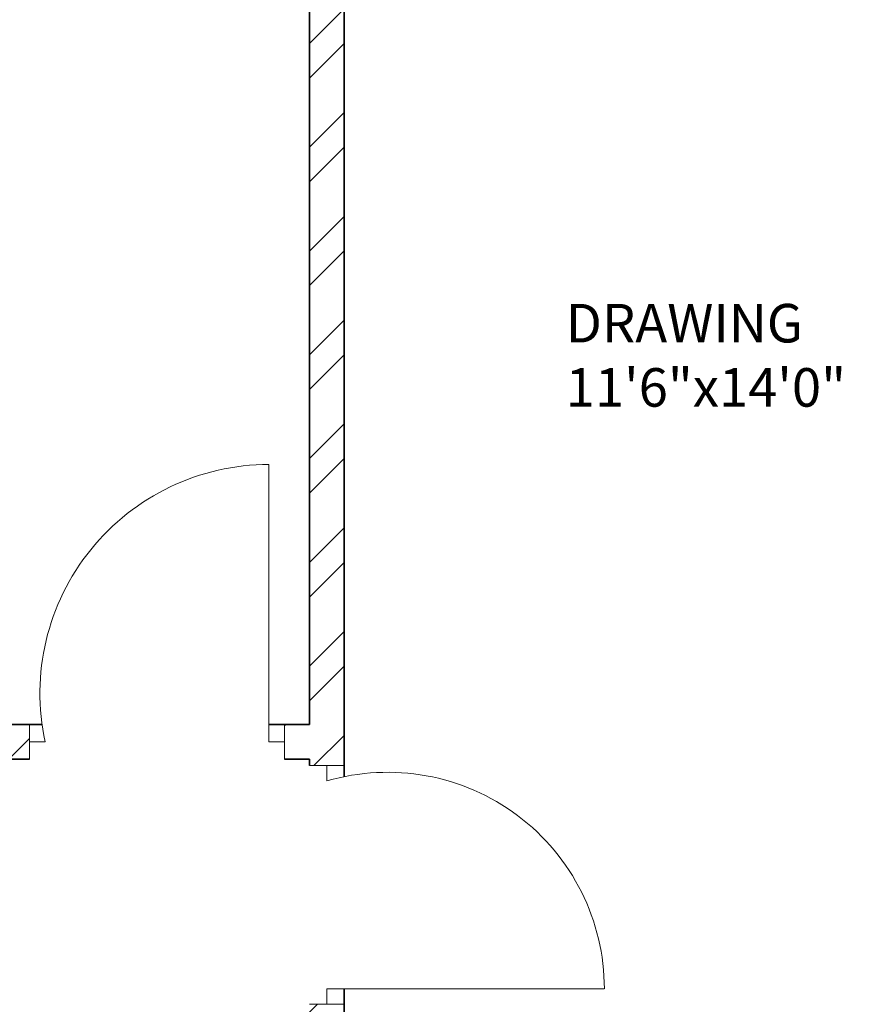
# Model space of a CAD drawing. Units: inches. Extents: x 1885 to 2748, y 783 to 2421.
# Tile 101 of 117: x 2449 to 2557, y 1850 to 1977. Entities that reach past the tile are written whole.
import ezdxf

# ---------------------------------------------------------------- set-up
doc = ezdxf.new("R2010")
doc.units = ezdxf.units.IN
for name, color, linetype, lineweight in [('A-AREA-IDEN', 7, 'Continuous', 18), ('A-DOOR', 31, 'Continuous', 18), ('A-WALL', 7, 'Continuous', 35)]:
    doc.layers.add(name, color=color, linetype=linetype, lineweight=lineweight)
doc.layers.add('A-WALL-PATT', color=85, linetype='Continuous', lineweight=13, true_color=0x58ba48)
doc.styles.get("Standard").update_dxf_attribs({"font": 'arial.ttf'})

msp = doc.modelspace()

# ---------------------------------------------------------------- hatches: boundary and pattern name
at = {"layer": 'A-WALL-PATT'}
h = msp.add_hatch(dxfattribs=at)
h.set_pattern_fill('ANSI32', color=256)
h.paths.add_polyline_path([(2007.77, 2318.01), (1980.77, 2318.01), (1980.77, 2281.22), (1985.27, 2281.22), (1985.27, 2313.51), (2007.77, 2313.51), (2007.77, 2315.76)])
h.paths.add_polyline_path([(2094.32, 2318.01), (2067.77, 2318.01), (2067.77, 2313.51), (2094.32, 2313.51), (2094.32, 2315.76)])
h.paths.add_polyline_path([(2131.37, 2315.76), (2131.37, 2318.01), (2131.19, 2318.01), (2112.61, 2318.01), (2112.61, 2313.51), (2117.27, 2313.51), (2117.27, 2255.2), (2121.77, 2255.2), (2121.77, 2313.51), (2131.37, 2313.51)])
h.paths.add_polyline_path([(2190.51, 2318.01), (2155.37, 2318.01), (2155.37, 2313.51), (2169.77, 2313.51), (2169.77, 2229.51), (2121.77, 2229.51), (2121.77, 2233.45), (2119.52, 2233.45), (2117.27, 2233.45), (2117.27, 2201.1), (2121.77, 2201.1), (2121.77, 2225.01), (2169.77, 2225.01), (2169.77, 2165.01), (2306.27, 2165.01), (2306.27, 2066.01), (2310.77, 2066.01), (2344.27, 2066.01), (2486.27, 2066.01), (2486.27, 1886.01), (2483.02, 1886.01), (2483.02, 1881.51), (2486.27, 1881.51), (2486.27, 1880.68), (2490.77, 1880.68), (2490.77, 2070.51), (2344.27, 2070.51), (2310.77, 2070.51), (2310.77, 2165.01), (2310.77, 2173.64), (2308.52, 2173.64), (2306.27, 2173.64), (2306.27, 2169.51), (2174.27, 2169.51), (2174.27, 2313.51), (2190.51, 2313.51), (2190.51, 2315.76)])
h.paths.add_polyline_path([(1985.27, 2221.22), (1980.77, 2221.22), (1980.77, 2165.01), (1992.77, 2165.01), (1992.77, 2141.93), (1997.27, 2141.93), (1997.27, 2165.01), (2117.27, 2165.01), (2117.27, 2163.13), (2121.77, 2163.13), (2121.77, 2172.73), (2119.52, 2172.73), (2117.27, 2172.73), (2117.27, 2169.51), (1985.27, 2169.51)])
h.paths.add_polyline_path([(1997.27, 2105.93), (1992.77, 2105.93), (1992.77, 2070.51), (2016.77, 2070.51), (2016.77, 2059.12), (2019.02, 2059.12), (2021.27, 2059.12), (2021.27, 2070.51), (2117.27, 2070.51), (2117.27, 2022.51), (2114.42, 2022.51), (2114.42, 2018.01), (2123.63, 2018.01), (2123.63, 2020.26), (2123.63, 2022.51), (2121.77, 2022.51), (2121.77, 2142.59), (2119.52, 2142.59), (2117.27, 2142.59), (2117.27, 2075.01), (1997.27, 2075.01)])
h.paths.add_polyline_path([(2092.03, 2020.26), (2092.03, 2022.51), (2021.27, 2022.51), (2021.27, 2035.12), (2016.77, 2035.12), (2016.77, 2018.01), (2016.77, 1978.78), (2021.27, 1978.78), (2021.27, 2018.01), (2092.03, 2018.01)])
h.paths.add_polyline_path([(2260.94, 2022.51), (2153.1, 2022.51), (2153.1, 2020.26), (2153.1, 2018.01), (2155.27, 2018.01), (2155.27, 1886.01), (2107.63, 1886.01), (2107.63, 1881.51), (2182.91, 1881.51), (2182.91, 1883.76), (2182.91, 1886.01), (2159.77, 1886.01), (2159.77, 2018.01), (2260.94, 2018.01), (2260.94, 2020.26)])
h.paths.add_polyline_path([(2047.63, 1883.76), (2047.63, 1886.01), (2021.27, 1886.01), (2021.27, 1918.78), (2019.02, 1918.78), (2016.77, 1918.78), (2016.77, 1881.51), (2047.63, 1881.51)])
h.paths.add_polyline_path([(2306.36, 1883.76), (2306.36, 1886.01), (2296.27, 1886.01), (2296.27, 1982.01), (2316.54, 1982.01), (2316.54, 1984.26), (2316.54, 1986.51), (2296.27, 1986.51), (2296.27, 2022.51), (2289.28, 2022.51), (2289.28, 2018.01), (2291.77, 2018.01), (2291.77, 1886.01), (2242.91, 1886.01), (2242.91, 1881.51), (2306.36, 1881.51)], flags=17)
h.paths.add_polyline_path([(1985.27, 1843.01), (2021.6, 1843.01), (2021.53, 1845.44), (2021.48, 1847.51), (1980.77, 1847.51), (1980.77, 1809.45), (1985.27, 1809.45)])
h.paths.add_polyline_path([(2131.48, 1845.26), (2131.48, 1847.51), (2081.53, 1847.51), (2081.53, 1843.01), (2117.27, 1843.01), (2117.27, 1784.15), (2119.52, 1784.15), (2121.77, 1784.15), (2121.77, 1843.01), (2131.48, 1843.01)])
h.paths.add_polyline_path([(2203.89, 1847.51), (2155.48, 1847.51), (2155.48, 1843.01), (2169.77, 1843.01), (2169.77, 1759.01), (2121.77, 1759.01), (2121.77, 1761.46), (2117.27, 1761.46), (2117.27, 1730.43), (2121.77, 1730.43), (2121.77, 1754.51), (2177.42, 1754.51), (2177.42, 1756.76), (2177.42, 1759.01), (2174.27, 1759.01), (2174.27, 1843.01), (2203.89, 1843.01)])
h.paths.add_polyline_path([(2335.55, 1845.26), (2335.55, 1847.51), (2239.89, 1847.51), (2239.89, 1843.01), (2306.27, 1843.01), (2306.27, 1759.01), (2199.49, 1759.01), (2199.49, 1754.51), (2310.77, 1754.51), (2310.77, 1843.01), (2335.55, 1843.01)])
h.paths.add_polyline_path([(2348.77, 2022.51), (2344.27, 2022.51), (2344.27, 1986.51), (2341.68, 1986.51), (2341.68, 1982.01), (2344.27, 1982.01), (2344.27, 1886.01), (2330.36, 1886.01), (2330.36, 1881.51), (2361.63, 1881.51), (2361.63, 1883.76), (2361.63, 1886.01), (2348.77, 1886.01)], flags=17)
h.paths.add_polyline_path([(2283.25, 2315.76), (2283.25, 2318.01), (2238.51, 2318.01), (2238.51, 2313.51), (2283.25, 2313.51)], flags=17)
h.paths.add_polyline_path([(2363.27, 2348.01), (2388.68, 2348.01), (2388.68, 2350.26), (2388.68, 2352.51), (2358.77, 2352.51), (2358.77, 2348.01), (2358.77, 2318.01), (2344.48, 2318.01), (2344.48, 2313.51), (2358.77, 2313.51), (2358.77, 2229.51), (2310.77, 2229.51), (2310.77, 2231.95), (2306.27, 2231.95), (2306.27, 2205.61), (2310.77, 2205.61), (2310.77, 2225.01), (2358.77, 2225.01), (2358.77, 2211.51), (2452.33, 2211.51), (2452.33, 2213.76), (2452.33, 2216.01), (2363.27, 2216.01), (2363.27, 2318.01)])
h.paths.add_polyline_path([(2310.77, 2313.51), (2320.48, 2313.51), (2320.48, 2315.76), (2320.48, 2318.01), (2302.73, 2318.01), (2302.73, 2313.51), (2306.27, 2313.51), (2306.27, 2251.08), (2310.77, 2251.08)], flags=17)
h.paths.add_polyline_path([(2490.77, 2352.51), (2486.27, 2352.51), (2448.68, 2352.51), (2448.68, 2348.01), (2486.27, 2348.01), (2486.27, 2318.01), (2486.27, 2216.01), (2481.78, 2216.01), (2481.78, 2211.51), (2486.27, 2211.51), (2486.27, 2165.01), (2493.29, 2165.01), (2493.29, 2167.26), (2493.29, 2169.51), (2490.77, 2169.51), (2490.77, 2313.51), (2494.43, 2313.51), (2494.43, 2318.01), (2490.77, 2318.01)])
h.paths.add_polyline_path([(2534.65, 2318.01), (2515.69, 2318.01), (2515.69, 2313.51), (2534.65, 2313.51), (2534.65, 2315.76)])
h.paths.add_polyline_path([(2618.27, 2318.01), (2594.65, 2318.01), (2594.65, 2313.51), (2613.77, 2313.51), (2613.77, 2281.71), (2618.27, 2281.71)])
h.paths.add_polyline_path([(2618.27, 2221.71), (2613.77, 2221.71), (2613.77, 2169.51), (2554.02, 2169.51), (2554.02, 2165.01), (2613.77, 2165.01), (2613.77, 2152.88), (2618.27, 2152.88)])
h.paths.add_polyline_path([(2618.27, 2128.88), (2616.02, 2128.88), (2613.77, 2128.88), (2613.77, 2117.01), (2529.77, 2117.01), (2529.77, 2165.01), (2532.85, 2165.01), (2532.85, 2169.51), (2522.87, 2169.51), (2522.87, 2165.01), (2525.27, 2165.01), (2525.27, 2117.01), (2525.27, 2112.51), (2525.27, 2108.58), (2529.77, 2108.58), (2529.77, 2112.51), (2613.77, 2112.51), (2613.77, 2080.19), (2618.27, 2080.19)])
h.paths.add_polyline_path([(2618.27, 2044.19), (2616.02, 2044.19), (2613.77, 2044.19), (2613.77, 2015.51), (2529.77, 2015.51), (2529.77, 2088.58), (2527.52, 2088.58), (2525.27, 2088.58), (2525.27, 2011.01), (2613.77, 2011.01), (2613.77, 1956.75), (2618.27, 1956.75)])
h.paths.add_polyline_path([(2618.27, 1881.51), (2618.27, 1896.75), (2613.77, 1896.75), (2613.77, 1881.51), (2613.77, 1847.51), (2592.71, 1847.51), (2592.71, 1843.01), (2613.77, 1843.01), (2613.77, 1765.01), (2613.77, 1760.51), (2609.62, 1760.51), (2609.62, 1756.01), (2613.77, 1756.01), (2613.77, 1660.01), (2608.54, 1660.01), (2608.54, 1655.51), (2613.77, 1655.51), (2613.77, 1508.16), (2618.27, 1508.16)])
h.paths.add_polyline_path([(2565.77, 1843.01), (2569, 1843.01), (2569, 1847.51), (2490.77, 1847.51), (2490.77, 1849.7), (2488.52, 1849.7), (2486.27, 1849.7), (2486.27, 1847.51), (2477.27, 1847.51), (2477.27, 1838.51), (2477.27, 1821.49), (2486.27, 1821.49), (2486.27, 1838.51), (2561.27, 1838.51), (2561.27, 1765.01), (2486.27, 1765.01), (2486.27, 1786.16), (2477.27, 1786.16), (2477.27, 1765.01), (2477.27, 1756.01), (2486.27, 1756.01), (2565.77, 1756.01), (2585.62, 1756.01), (2585.62, 1758.26), (2585.62, 1760.51), (2565.77, 1760.51), (2565.77, 1765.01)])
h.paths.add_polyline_path([(2486.27, 1651.01), (2561.27, 1651.01), (2561.27, 1567.01), (2486.27, 1567.01), (2486.27, 1591.32), (2477.27, 1591.32), (2477.27, 1567.01), (2477.27, 1558.01), (2477.27, 1555.44), (2481.77, 1555.44), (2481.77, 1558.01), (2568.65, 1558.01), (2568.65, 1560.26), (2568.65, 1562.51), (2565.77, 1562.51), (2565.77, 1655.51), (2584.54, 1655.51), (2584.54, 1657.76), (2584.54, 1660.01), (2565.77, 1660.01), (2486.27, 1660.01), (2477.27, 1660.01), (2477.27, 1651.01), (2477.27, 1632.99), (2486.27, 1632.99)])
h.paths.add_polyline_path([(2449.97, 1883.76), (2449.97, 1886.01), (2421.63, 1886.01), (2421.63, 1881.51), (2449.97, 1881.51)], flags=17)
h.paths.add_polyline_path([(2447.27, 1847.51), (2395.55, 1847.51), (2395.55, 1843.01), (2442.77, 1843.01), (2442.77, 1809.27), (2447.27, 1809.27)])
h.paths.add_polyline_path([(1985.27, 1749.45), (1980.77, 1749.45), (1980.77, 1694.5), (1985.27, 1694.5), (1985.27, 1694.51), (1986.9, 1694.51), (1986.9, 1697.78), (1986.9, 1699.01), (1985.27, 1699.01)])
h.paths.add_polyline_path([(2152.77, 1699.01), (2121.77, 1699.01), (2121.77, 1703.67), (2119.52, 1703.67), (2117.27, 1703.67), (2117.27, 1699.01), (2009.22, 1699.01), (2009.22, 1694.51), (2148.27, 1694.51), (2148.27, 1692.63), (2152.77, 1692.63)])
h.paths.add_polyline_path([(2016.27, 1694.51), (2011.77, 1694.51), (2011.77, 1558.01), (2040.81, 1558.01), (2040.81, 1560.26), (2040.81, 1562.51), (2016.27, 1562.51)])
h.paths.add_polyline_path([(2152.77, 1663.02), (2150.52, 1663.02), (2148.27, 1663.02), (2148.27, 1562.51), (2100.81, 1562.51), (2100.81, 1558.01), (2165.12, 1558.01), (2165.12, 1560.26), (2165.12, 1562.51), (2152.77, 1562.51), (2152.77, 1610.51), (2224.77, 1610.51), (2224.77, 1607.99), (2229.27, 1607.99), (2229.27, 1615.01), (2152.77, 1615.01)])
h.paths.add_polyline_path([(2238.61, 1560.26), (2238.61, 1562.51), (2229.27, 1562.51), (2229.27, 1588.76), (2227.02, 1588.76), (2224.77, 1588.77), (2224.77, 1562.51), (2189.12, 1562.51), (2189.12, 1558.01), (2238.61, 1558.01)])
h.paths.add_polyline_path([(2336.02, 1560.26), (2336.02, 1562.51), (2310.77, 1562.51), (2310.77, 1656.35), (2308.52, 1656.35), (2306.27, 1656.35), (2306.27, 1562.51), (2286.61, 1562.51), (2286.61, 1558.01), (2336.02, 1558.01)])
h.paths.add_polyline_path([(2447.27, 1690.97), (2445.02, 1690.97), (2442.77, 1690.97), (2442.77, 1687.01), (2306.27, 1687.01), (2306.27, 1680.75), (2310.77, 1680.75), (2310.77, 1682.51), (2442.77, 1682.51), (2442.77, 1562.51), (2396.02, 1562.51), (2396.02, 1558.01), (2447.27, 1558.01)])
h.paths.add_polyline_path([(2447.27, 1749.27), (2445.02, 1749.27), (2442.77, 1749.27), (2442.77, 1717.23), (2447.27, 1717.23)])
h.paths.add_polyline_path([(2044.67, 1521.76), (2044.67, 1524.01), (2007.27, 1524.01), (2007.27, 1503.49), (2009.52, 1503.49), (2011.77, 1503.49), (2011.77, 1519.51), (2044.67, 1519.51)])
h.paths.add_polyline_path([(2177.97, 1521.76), (2177.97, 1524.01), (2104.67, 1524.01), (2104.67, 1519.51), (2145.77, 1519.51), (2145.77, 1387.51), (2143.37, 1387.51), (2143.37, 1383.01), (2251.59, 1383.01), (2251.59, 1385.26), (2251.59, 1387.51), (2150.27, 1387.51), (2150.27, 1519.51), (2177.97, 1519.51)])
h.paths.add_polyline_path([(2298.7, 1524.01), (2237.97, 1524.01), (2237.97, 1519.51), (2282.27, 1519.51), (2282.27, 1387.51), (2279.68, 1387.51), (2279.68, 1383.01), (2286.77, 1383.01), (2286.77, 1419.01), (2312.45, 1419.01), (2312.45, 1421.26), (2312.45, 1423.51), (2286.77, 1423.51), (2286.77, 1519.51), (2298.7, 1519.51), (2298.7, 1521.72)], flags=17)
h.paths.add_polyline_path([(2361.9, 1521.76), (2361.9, 1524.01), (2322.7, 1524.01), (2322.7, 1519.51), (2334.77, 1519.51), (2334.77, 1423.51), (2331.93, 1423.51), (2331.93, 1419.01), (2334.77, 1419.01), (2334.77, 1387.51), (2334.77, 1383.23), (2339.27, 1383.23), (2339.27, 1387.51), (2339.27, 1519.51), (2361.9, 1519.51)], flags=17)
h.paths.add_polyline_path([(2447.27, 1521.76), (2447.27, 1524.01), (2421.9, 1524.01), (2421.9, 1519.51), (2447.27, 1519.51)], flags=17)
h.paths.add_polyline_path([(2481.77, 1529.6), (2479.52, 1529.6), (2477.27, 1529.6), (2477.27, 1524.01), (2474.49, 1524.01), (2474.49, 1519.51), (2477.27, 1519.51), (2477.27, 1334.51), (2296.77, 1334.51), (2296.77, 1240.51), (2160.27, 1240.51), (2160.27, 1180.51), (2112.27, 1180.51), (2112.27, 1207.69), (2110.02, 1207.69), (2107.77, 1207.69), (2107.77, 1171.61), (2112.27, 1171.61), (2112.27, 1176.01), (2160.27, 1176.01), (2160.27, 1092.01), (2144.22, 1092.01), (2144.22, 1087.51), (2189.5, 1087.51), (2189.5, 1089.76), (2189.5, 1092.01), (2164.77, 1092.01), (2164.77, 1236.01), (2296.77, 1236.01), (2296.77, 1231.91), (2301.27, 1231.91), (2301.27, 1330.01), (2481.77, 1330.01), (2481.77, 1387.51)])
h.paths.add_polyline_path([(2618.27, 1448.16), (2613.77, 1448.16), (2613.77, 1382.51), (2529.77, 1382.51), (2525.27, 1382.51), (2525.27, 1307.06), (2529.77, 1307.06), (2529.77, 1378.01), (2613.77, 1378.01), (2613.77, 1354.99), (2618.27, 1354.99)])
h.paths.add_polyline_path([(2618.27, 1318.99), (2613.77, 1318.99), (2613.77, 1281.01), (2529.77, 1281.01), (2529.77, 1283.79), (2527.52, 1283.79), (2525.27, 1283.79), (2525.27, 1228.51), (2516.79, 1228.51), (2516.79, 1224.01), (2533.48, 1224.01), (2533.48, 1226.26), (2533.48, 1228.51), (2529.77, 1228.51), (2529.77, 1276.51), (2613.77, 1276.51), (2613.77, 1266.02), (2618.27, 1266.02)])
h.paths.add_polyline_path([(2618.27, 1134.96), (2613.77, 1134.96), (2613.77, 1092.01), (2594.54, 1092.01), (2594.54, 1087.51), (2618.27, 1087.51)])
h.paths.add_polyline_path([(2534.54, 1092.01), (2509.77, 1092.01), (2509.77, 1087.51), (2534.54, 1087.51), (2534.54, 1089.76)])
h.paths.add_polyline_path([(2481.27, 1224.01), (2484.12, 1224.01), (2484.12, 1226.26), (2484.12, 1228.51), (2476.77, 1228.51), (2476.77, 1198.51), (2471.61, 1198.51), (2471.61, 1194.01), (2476.77, 1194.01), (2476.77, 1062.01), (2436.89, 1062.01), (2436.89, 1057.51), (2476.77, 1057.51), (2481.27, 1057.51), (2481.27, 1062.01), (2481.27, 1087.51), (2485.35, 1087.51), (2485.35, 1089.76), (2485.35, 1092.01), (2481.27, 1092.01), (2481.27, 1117.51)])
h.paths.add_polyline_path([(2439.9, 1198.51), (2349.27, 1198.51), (2349.27, 1194.01), (2349.27, 1180.51), (2301.27, 1180.51), (2301.27, 1201.9), (2299.02, 1201.9), (2296.77, 1201.9), (2296.77, 1172.34), (2299.02, 1172.34), (2301.27, 1172.34), (2301.27, 1176.01), (2349.27, 1176.01), (2349.27, 1092.01), (2334.45, 1092.01), (2334.45, 1087.51), (2349.27, 1087.51), (2349.27, 1057.51), (2353.77, 1057.51), (2376.89, 1057.51), (2376.89, 1059.76), (2376.89, 1062.01), (2353.77, 1062.01), (2353.77, 1087.51), (2353.77, 1180.51), (2353.77, 1194.01), (2439.9, 1194.01), (2439.9, 1196.26)])
h.paths.add_polyline_path([(2270.6, 1089.76), (2270.6, 1092.01), (2249.5, 1092.01), (2249.5, 1087.51), (2270.6, 1087.51)], flags=17)
h.paths.add_polyline_path([(2310.45, 1092.01), (2301.27, 1092.01), (2301.27, 1153.29), (2296.77, 1153.29), (2296.77, 1092.01), (2293.79, 1092.01), (2293.79, 1087.51), (2310.45, 1087.51), (2310.45, 1089.76)], flags=17)
h.paths.add_polyline_path([(2112.27, 1150.33), (2110.02, 1150.33), (2107.77, 1150.33), (2107.77, 1092.01), (2104.47, 1092.01), (2104.47, 1087.51), (2120.22, 1087.51), (2120.22, 1089.76), (2120.22, 1092.01), (2112.27, 1092.01)])
h.paths.add_polyline_path([(2082.17, 1092.01), (2058.14, 1092.01), (2058.14, 1087.51), (2082.17, 1087.51), (2082.17, 1089.76)])
h.paths.add_polyline_path([(1975.77, 1145.64), (1971.27, 1145.64), (1971.27, 1087.51), (1980.77, 1087.51), (1998.14, 1087.51), (1998.14, 1089.76), (1998.14, 1092.01), (1985.27, 1092.01), (1975.77, 1092.01)])
h.paths.add_polyline_path([(2112.27, 1244.38), (2110.02, 1244.38), (2107.77, 1244.38), (2107.77, 1240.51), (1992.27, 1240.51), (1992.27, 1271.01), (1987.77, 1271.01), (1987.77, 1240.51), (1980.77, 1240.51), (1975.77, 1240.51), (1971.27, 1240.51), (1971.27, 1205.64), (1975.77, 1205.64), (1975.77, 1236.01), (2107.77, 1236.01), (2107.77, 1233.44), (2112.27, 1233.44), (2112.27, 1236.01)])
h.paths.add_polyline_path([(2112.27, 1383.01), (2114.78, 1383.01), (2114.78, 1385.26), (2114.78, 1387.51), (2102.48, 1387.51), (2102.48, 1383.01), (2107.77, 1383.01), (2107.77, 1335.01), (2011.77, 1335.01), (2011.77, 1349.94), (2007.27, 1349.94), (2007.27, 1335.01), (1987.77, 1335.01), (1987.77, 1330.51), (1987.77, 1307.01), (1992.27, 1307.01), (1992.27, 1330.51), (2007.27, 1330.51), (2107.77, 1330.51), (2107.77, 1264.71), (2112.27, 1264.71)])
h.paths.add_polyline_path([(2077.86, 1387.51), (2011.77, 1387.51), (2011.77, 1390.04), (2009.52, 1390.04), (2007.27, 1390.04), (2007.27, 1373.94), (2011.77, 1373.94), (2011.77, 1383.01), (2077.86, 1383.01)])
h.paths.add_polyline_path([(2011.77, 1443.49), (2007.27, 1443.49), (2007.27, 1410.25), (2011.77, 1410.25)])

# ---------------------------------------------------------------- linework, layer by layer
at = {"layer": 'A-DOOR'}
for p, q in [((2481.02, 1883.76), (2481.02, 1919.76)), ((2449.97, 1886.01), (2449.97, 1881.51)), ((2483.02, 1886.01), (2483.02, 1881.51)), ((2449.97, 1881.51), (2449.97, 1883.76)), ((2449.97, 1883.76), (2451.97, 1883.76)), ((2483.02, 1883.76), (2481.02, 1883.76)), ((2483.02, 1881.51), (2483.02, 1883.76)), ((2486.27, 1880.68), (2490.77, 1880.68)), ((2490.77, 1880.68), (2488.52, 1880.68)), ((2488.52, 1880.68), (2488.52, 1878.68)), ((2488.52, 1849.7), (2488.52, 1851.7)), ((2488.52, 1851.7), (2524.52, 1851.7)), ((2486.27, 1849.7), (2490.77, 1849.7)), ((2490.77, 1849.7), (2488.52, 1849.7))]:
    msp.add_line(p, q, dxfattribs=at)
for centre, radius, start, end in [((2481.02, 1890.03), 29.72, 90, 192.1907), ((2496.42, 1851.7), 28.11, 0, 106.3054)]:
    msp.add_arc(centre, radius, start, end, dxfattribs=at)
at = {"layer": 'A-WALL'}
for p, q in [((2490.77, 2070.51), (2490.77, 1879.24)), ((2486.27, 2066.01), (2486.27, 1886.01)), ((2451.57, 1886.01), (2421.63, 1886.01)), ((2486.27, 1886.01), (2481.02, 1886.01)), ((2421.63, 1881.51), (2449.97, 1881.51)), ((2483.02, 1881.51), (2486.27, 1881.51)), ((2486.27, 1881.51), (2486.27, 1880.68)), ((2490.77, 1851.7), (2490.77, 1847.51))]:
    msp.add_line(p, q, dxfattribs=at)

# ---------------------------------------------------------------- texts
at = {"layer": 'A-AREA-IDEN', "insert": (2519.52, 1940.59), "char_height": 5, "attachment_point": 1}
msp.add_mtext_dynamic_manual_height_columns('DRAWING\\P11\'6"x14\'0"', width=207.0969, gutter_width=12.5, heights=[0], dxfattribs=at)

doc.saveas('drawing.dxf')
